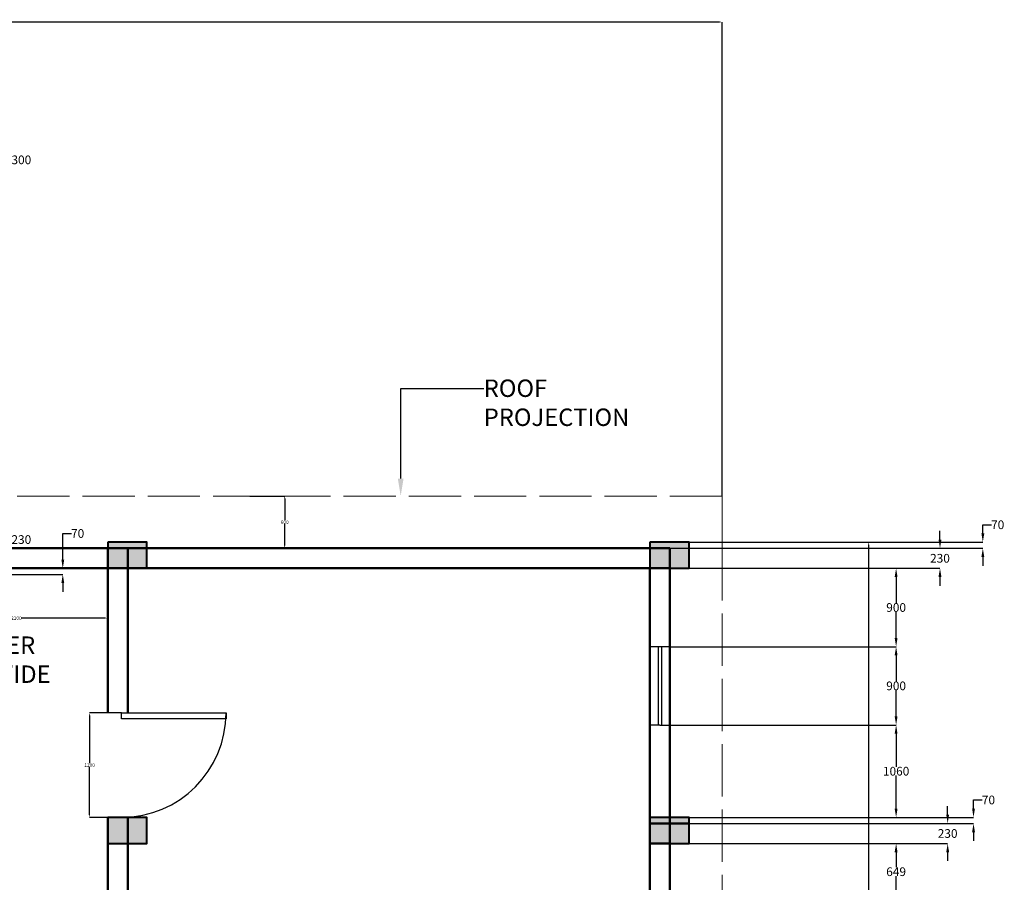
# Model space of a CAD drawing. Units: millimetres. Extents: x -17156 to 39375, y -45872 to -24892.
# Tile 11 of 12: x 5351 to 16665, y -35444 to -25539. Entities that reach past the tile are written whole.
import ezdxf
from ezdxf import colors
from ezdxf.entities.mleader import LeaderData, LeaderLine
from ezdxf.math import Vec2, Vec3

# ---------------------------------------------------------------- set-up
doc = ezdxf.new("R2010")
doc.units = ezdxf.units.MM
doc.header["$MEASUREMENT"] = 0
doc.linetypes.add('ACAD_ISO02W100', pattern=[15, 12, -3])
for name, color, linetype, lineweight in [('A-ANNO-DIMS', 2, 'Continuous', 18), ('A-ANNO-TEXT', 4, 'Continuous', 18), ('A-AREA-IDEN', 4, 'Continuous', 25), ('A-COLS', 7, 'Continuous', 40), ('A-ROOF-OVHD', 8, 'ACAD_ISO02W100', 18), ('DOORS', 6, 'Continuous', 25), ('WALLS', 5, 'Continuous', 50), ('WINDOW', 240, 'Continuous', 25)]:
    doc.layers.add(name, color=color, linetype=linetype, lineweight=lineweight)
doc.styles.get("Standard").update_dxf_attribs({"font": 'arial.ttf'})
doc.dimstyles.get("Standard").update_dxf_attribs({"dimtxt": 40, "dimasz": 30.18, "dimexe": 0, "dimexo": 0.0625, "dimgap": 0.09, "dimtad": 0, "dimtih": 1, "dimtoh": 1, "dimdec": 0, "dimzin": 0, "dimdsep": 46, "dimtxsty": 'Standard', "dimcen": 0.09, "dimadec": 0, "dimazin": 0, "dimtfac": 1, "dimtdec": 0, "dimtofl": 0, "dimtmove": 0, "dimatfit": 3, "dimfxl": 1, "dimtolj": 1, "dimtzin": 0, "dimarcsym": 0})

# ---------------------------------------------------------------- blocks, each defined once
blk = doc.blocks.new('*U8')
for p, q in [((-750, 0), (-750, 100)), ((0, 0), (0, 100))]:
    blk.add_line(p, q)
blk.add_lwpolyline([(0, 0), (0, -750), (-43.75, -750), (-43.75, 0)], close=True)
blk.add_arc((0, 0), 750, 180, 270)
blk = doc.blocks.new('*D44')
at = {"layer": 'A-ANNO-DIMS', "color": 0, "lineweight": -2, "transparency": 16777216}
for p, q in [((13043, -34998), (15422, -34998)), ((15422, -35098), (15422, -35271)), ((15422, -35547), (15422, -35374)), ((12823, -35647), (15422, -35647))]:
    blk.add_line(p, q, dxfattribs=at)
at = {"layer": 'A-ANNO-DIMS', "color": 0, "lineweight": 100, "transparency": 16777216}
for points in [[(15405, -35098), (15438, -35098), (15422, -34998)], [(15405, -35547), (15438, -35547), (15422, -35647)]]:
    blk.add_solid(points, dxfattribs=at)
at = {"layer": 'Defpoints', "color": 0, "lineweight": 100, "transparency": 16777216}
for p in [(13043, -34998), (15422, -34998), (12823, -35647)]:
    blk.add_point(p, dxfattribs=at)
at = {"layer": 'A-ANNO-DIMS', "color": 0, "transparency": 16777216, "insert": (15422, -35322), "char_height": 100, "attachment_point": 5}
blk.add_mtext('\\A1;649', dxfattribs=at)
blk = doc.blocks.new('*D45')
at = {"layer": 'A-ANNO-DIMS', "color": 0, "lineweight": -2, "transparency": 16777216}
for p, q in [((16014, -34668), (16014, -34568)), ((13043, -34768), (16014, -34768)), ((13043, -34998), (16014, -34998)), ((16014, -35098), (16014, -35198))]:
    blk.add_line(p, q, dxfattribs=at)
at = {"layer": 'A-ANNO-DIMS', "color": 0, "lineweight": 100, "transparency": 16777216}
for points in [[(15998, -34668), (16031, -34668), (16014, -34768)], [(15998, -35098), (16031, -35098), (16014, -34998)]]:
    blk.add_solid(points, dxfattribs=at)
at = {"layer": 'Defpoints', "color": 0, "lineweight": 100, "transparency": 16777216}
for p in [(13043, -34768), (16014, -34768), (13043, -34998)]:
    blk.add_point(p, dxfattribs=at)
at = {"layer": 'A-ANNO-DIMS', "color": 0, "transparency": 16777216, "insert": (16014, -34883), "char_height": 100, "attachment_point": 5}
blk.add_mtext('\\A1;230', dxfattribs=at)
blk = doc.blocks.new('*D46')
at = {"layer": 'A-ANNO-DIMS', "color": 0, "lineweight": -2, "transparency": 16777216}
for p, q in [((16311, -34598), (16311, -34498)), ((16311, -34498), (16411, -34498)), ((13043, -34698), (16311, -34698)), ((13043, -34768), (16311, -34768)), ((16311, -34868), (16311, -34968))]:
    blk.add_line(p, q, dxfattribs=at)
at = {"layer": 'A-ANNO-DIMS', "color": 0, "lineweight": 100, "transparency": 16777216}
for points in [[(16295, -34598), (16328, -34598), (16311, -34698)], [(16295, -34868), (16328, -34868), (16311, -34768)]]:
    blk.add_solid(points, dxfattribs=at)
at = {"layer": 'Defpoints', "color": 0, "lineweight": 100, "transparency": 16777216}
for p in [(13043, -34698), (16311, -34698), (13043, -34768)]:
    blk.add_point(p, dxfattribs=at)
at = {"layer": 'A-ANNO-DIMS', "color": 0, "transparency": 16777216, "insert": (16483, -34498), "char_height": 100, "attachment_point": 5}
blk.add_mtext('\\A1;70', dxfattribs=at)
blk = doc.blocks.new('*D47')
at = {"layer": 'A-ANNO-DIMS', "color": 0, "lineweight": -2, "transparency": 16777216}
for p, q in [((12823, -33638), (15422, -33638)), ((15422, -33738), (15422, -34117)), ((15422, -34598), (15422, -34219)), ((13043, -34698), (15422, -34698))]:
    blk.add_line(p, q, dxfattribs=at)
at = {"layer": 'A-ANNO-DIMS', "color": 0, "lineweight": 100, "transparency": 16777216}
for points in [[(15405, -33738), (15438, -33738), (15422, -33638)], [(15405, -34598), (15438, -34598), (15422, -34698)]]:
    blk.add_solid(points, dxfattribs=at)
at = {"layer": 'Defpoints', "color": 0, "lineweight": 100, "transparency": 16777216}
for p in [(12823, -33638), (15422, -33638), (13043, -34698)]:
    blk.add_point(p, dxfattribs=at)
at = {"layer": 'A-ANNO-DIMS', "color": 0, "transparency": 16777216, "insert": (15422, -34168), "char_height": 100, "attachment_point": 5}
blk.add_mtext('\\A1;1060', dxfattribs=at)
blk = doc.blocks.new('*D48')
at = {"layer": 'A-ANNO-DIMS', "color": 0, "lineweight": -2, "transparency": 16777216}
for p, q in [((12823, -32738), (15422, -32738)), ((15422, -32838), (15422, -33136)), ((15422, -33538), (15422, -33239)), ((12823, -33638), (15422, -33638))]:
    blk.add_line(p, q, dxfattribs=at)
at = {"layer": 'A-ANNO-DIMS', "color": 0, "lineweight": 100, "transparency": 16777216}
for points in [[(15405, -32838), (15438, -32838), (15422, -32738)], [(15405, -33538), (15438, -33538), (15422, -33638)]]:
    blk.add_solid(points, dxfattribs=at)
at = {"layer": 'Defpoints', "color": 0, "lineweight": 100, "transparency": 16777216}
for p in [(12823, -32738), (15422, -32738), (12823, -33638)]:
    blk.add_point(p, dxfattribs=at)
at = {"layer": 'A-ANNO-DIMS', "color": 0, "transparency": 16777216, "insert": (15422, -33188), "char_height": 100, "attachment_point": 5}
blk.add_mtext('\\A1;900', dxfattribs=at)
blk = doc.blocks.new('*D49')
at = {"layer": 'A-ANNO-DIMS', "color": 0, "lineweight": -2, "transparency": 16777216}
for p, q in [((13043, -31838), (15422, -31838)), ((15422, -31938), (15422, -32237)), ((15422, -32638), (15422, -32339)), ((12823, -32738), (15422, -32738))]:
    blk.add_line(p, q, dxfattribs=at)
at = {"layer": 'A-ANNO-DIMS', "color": 0, "lineweight": 100, "transparency": 16777216}
for points in [[(15405, -31938), (15438, -31938), (15422, -31838)], [(15405, -32638), (15438, -32638), (15422, -32738)]]:
    blk.add_solid(points, dxfattribs=at)
at = {"layer": 'Defpoints', "color": 0, "lineweight": 100, "transparency": 16777216}
for p in [(13043, -31838), (15422, -31838), (12823, -32738)]:
    blk.add_point(p, dxfattribs=at)
at = {"layer": 'A-ANNO-DIMS', "color": 0, "transparency": 16777216, "insert": (15422, -32288), "char_height": 100, "attachment_point": 5}
blk.add_mtext('\\A1;900', dxfattribs=at)
blk = doc.blocks.new('*D50')
at = {"layer": 'A-ANNO-DIMS', "color": 0, "lineweight": -2, "transparency": 16777216}
for p, q in [((15926, -31508), (15926, -31408)), ((12823, -31608), (15926, -31608)), ((13043, -31838), (15926, -31838)), ((15926, -31938), (15926, -32038))]:
    blk.add_line(p, q, dxfattribs=at)
at = {"layer": 'A-ANNO-DIMS', "color": 0, "lineweight": 100, "transparency": 16777216}
for points in [[(15909, -31508), (15943, -31508), (15926, -31608)], [(15909, -31938), (15943, -31938), (15926, -31838)]]:
    blk.add_solid(points, dxfattribs=at)
at = {"layer": 'Defpoints', "color": 0, "lineweight": 100, "transparency": 16777216}
for p in [(12823, -31608), (15926, -31608), (13043, -31838)]:
    blk.add_point(p, dxfattribs=at)
at = {"layer": 'A-ANNO-DIMS', "color": 0, "transparency": 16777216, "insert": (15926, -31723), "char_height": 100, "attachment_point": 5}
blk.add_mtext('\\A1;230', dxfattribs=at)
blk = doc.blocks.new('*D51')
at = {"layer": 'A-ANNO-DIMS', "color": 0, "lineweight": -2, "transparency": 16777216}
for p, q in [((16418, -31438), (16418, -31338)), ((16418, -31338), (16518, -31338)), ((13043, -31538), (16418, -31538)), ((12823, -31608), (16418, -31608)), ((16418, -31708), (16418, -31808))]:
    blk.add_line(p, q, dxfattribs=at)
at = {"layer": 'A-ANNO-DIMS', "color": 0, "lineweight": 100, "transparency": 16777216}
for points in [[(16402, -31438), (16435, -31438), (16418, -31538)], [(16402, -31708), (16435, -31708), (16418, -31608)]]:
    blk.add_solid(points, dxfattribs=at)
at = {"layer": 'Defpoints', "color": 0, "lineweight": 100, "transparency": 16777216}
for p in [(13043, -31538), (16418, -31538), (12823, -31608)]:
    blk.add_point(p, dxfattribs=at)
at = {"layer": 'A-ANNO-DIMS', "color": 0, "transparency": 16777216, "insert": (16589, -31338), "char_height": 100, "attachment_point": 5}
blk.add_mtext('\\A1;70', dxfattribs=at)
blk = doc.blocks.new('*D73')
at = {"layer": 'A-ANNO-DIMS', "color": 0, "lineweight": -2, "transparency": 16777216}
for p, q in [((5846, -31738), (5846, -31438)), ((5846, -31438), (5946, -31438)), ((4493, -31838), (5846, -31838)), ((4493, -31908), (5846, -31908)), ((5846, -32008), (5846, -32108))]:
    blk.add_line(p, q, dxfattribs=at)
at = {"layer": 'A-ANNO-DIMS', "color": 0, "lineweight": 100, "transparency": 16777216}
for points in [[(5830, -31738), (5863, -31738), (5846, -31838)], [(5830, -32008), (5863, -32008), (5846, -31908)]]:
    blk.add_solid(points, dxfattribs=at)
at = {"layer": 'Defpoints', "color": 0, "lineweight": 100, "transparency": 16777216}
for p in [(4493, -31838), (5846, -31838), (4493, -31908)]:
    blk.add_point(p, dxfattribs=at)
at = {"layer": 'A-ANNO-DIMS', "color": 0, "transparency": 16777216, "insert": (6017, -31438), "char_height": 100, "attachment_point": 5}
blk.add_mtext('\\A1;70', dxfattribs=at)
blk = doc.blocks.new('*D74')
at = {"layer": 'A-ANNO-DIMS', "color": 0, "lineweight": -2, "transparency": 16777216}
for p, q in [((5159, -31608), (5159, -31508)), ((5159, -31508), (5259, -31508)), ((4493, -31608), (5159, -31608)), ((5159, -31738), (5159, -31708)), ((4493, -31838), (5159, -31838))]:
    blk.add_line(p, q, dxfattribs=at)
at = {"layer": 'A-ANNO-DIMS', "color": 0, "lineweight": 100, "transparency": 16777216}
for points in [[(5143, -31708), (5176, -31708), (5159, -31608)], [(5143, -31738), (5176, -31738), (5159, -31838)]]:
    blk.add_solid(points, dxfattribs=at)
at = {"layer": 'Defpoints', "color": 0, "lineweight": 100, "transparency": 16777216}
for p in [(4493, -31608), (5159, -31608), (4493, -31838)]:
    blk.add_point(p, dxfattribs=at)
at = {"layer": 'A-ANNO-DIMS', "color": 0, "transparency": 16777216, "insert": (5370, -31508), "char_height": 100, "attachment_point": 5}
blk.add_mtext('\\A1;230', dxfattribs=at)
blk = doc.blocks.new('*D76')
at = {"layer": 'A-ANNO-DIMS', "color": 0, "lineweight": -2, "transparency": 16777216}
for p, q in [((5159, -27248), (5159, -27148)), ((5159, -27148), (5259, -27148)), ((4493, -27248), (5159, -27248)), ((5159, -27448), (5159, -27348)), ((4493, -27548), (5159, -27548))]:
    blk.add_line(p, q, dxfattribs=at)
at = {"layer": 'A-ANNO-DIMS', "color": 0, "lineweight": 100, "transparency": 16777216}
for points in [[(5143, -27348), (5176, -27348), (5159, -27248)], [(5143, -27448), (5176, -27448), (5159, -27548)]]:
    blk.add_solid(points, dxfattribs=at)
at = {"layer": 'Defpoints', "color": 0, "lineweight": 100, "transparency": 16777216}
for p in [(4493, -27248), (5159, -27248), (4493, -27548)]:
    blk.add_point(p, dxfattribs=at)
at = {"layer": 'A-ANNO-DIMS', "color": 0, "transparency": 16777216, "insert": (5370, -27148), "char_height": 100, "attachment_point": 5}
blk.add_mtext('\\A1;300', dxfattribs=at)
blk = doc.blocks.new('*D107')
at = {"layer": 'A-ANNO-DIMS', "color": 0, "lineweight": -2, "transparency": 16777216}
for p, q in [((4263, -31890), (4263, -32410)), ((6363, -31890), (6363, -32410)), ((4293, -32410), (5253, -32410)), ((6332, -32410), (5373, -32410))]:
    blk.add_line(p, q, dxfattribs=at)
at = {"layer": 'A-ANNO-DIMS', "color": 0, "lineweight": 100, "transparency": 16777216}
for points in [[(4293, -32405), (4293, -32415), (4263, -32410)], [(6332, -32405), (6332, -32415), (6363, -32410)]]:
    blk.add_solid(points, dxfattribs=at)
at = {"layer": 'Defpoints', "color": 0, "lineweight": 100, "transparency": 16777216}
for p in [(4263, -31890), (6363, -31890), (6363, -32410)]:
    blk.add_point(p, dxfattribs=at)
at = {"layer": 'A-ANNO-DIMS', "color": 0, "transparency": 16777216, "insert": (5313, -32410), "char_height": 40, "attachment_point": 5}
blk.add_mtext('\\A1;2100', dxfattribs=at)
blk = doc.blocks.new('*D110')
at = {"layer": 'A-ANNO-DIMS', "color": 0, "lineweight": -2, "transparency": 16777216}
for p, q in [((7996, -31008), (8396, -31008)), ((8396, -31038), (8396, -31287)), ((8396, -31578), (8396, -31328)), ((7996, -31608), (8396, -31608))]:
    blk.add_line(p, q, dxfattribs=at)
at = {"layer": 'A-ANNO-DIMS', "color": 0, "lineweight": 100, "transparency": 16777216}
for points in [[(8391, -31038), (8401, -31038), (8396, -31008)], [(8391, -31578), (8401, -31578), (8396, -31608)]]:
    blk.add_solid(points, dxfattribs=at)
at = {"layer": 'Defpoints', "color": 0, "lineweight": 100, "transparency": 16777216}
for p in [(7996, -31008), (7996, -31608), (8396, -31608)]:
    blk.add_point(p, dxfattribs=at)
at = {"layer": 'A-ANNO-DIMS', "color": 0, "transparency": 16777216, "insert": (8396, -31308), "char_height": 40, "attachment_point": 5}
blk.add_mtext('\\A1;600', dxfattribs=at)
blk = doc.blocks.new('*D113')
at = {"layer": 'A-ANNO-DIMS', "color": 0, "lineweight": -2, "transparency": 16777216}
for p, q in [((6363, -33498), (6155, -33498)), ((6155, -33528), (6155, -34077)), ((6155, -34668), (6155, -34118)), ((6363, -34698), (6155, -34698))]:
    blk.add_line(p, q, dxfattribs=at)
at = {"layer": 'A-ANNO-DIMS', "color": 0, "lineweight": 100, "transparency": 16777216}
for points in [[(6150, -33528), (6160, -33528), (6155, -33498)], [(6150, -34668), (6160, -34668), (6155, -34698)]]:
    blk.add_solid(points, dxfattribs=at)
at = {"layer": 'Defpoints', "color": 0, "lineweight": 100, "transparency": 16777216}
for p in [(6363, -33498), (6155, -34698), (6363, -34698)]:
    blk.add_point(p, dxfattribs=at)
at = {"layer": 'A-ANNO-DIMS', "color": 0, "transparency": 16777216, "insert": (6155, -34098), "char_height": 40, "attachment_point": 5}
blk.add_mtext('\\A1;1200', dxfattribs=at)
blk = doc.blocks.new('WIN-900x230')
for p, q in [((0, 900), (230, 900)), ((95, 900), (95, 0)), ((135, 900), (135, 0)), ((115, 0), (0, 0)), ((115, 0), (230, 0))]:
    blk.add_line(p, q)
blk = doc.blocks.new('COL-450x300')
h = blk.add_hatch(color=256)
h.dxf.hatch_style = 1
h.paths.add_polyline_path([(0, 300), (0, 0), (450, 0), (450, 300)])
blk.add_lwpolyline([(0, 300), (0, 0), (450, 0), (450, 300)], close=True)
blk = doc.blocks.new('*D144')
at = {"layer": 'A-ANNO-DIMS', "color": 0, "lineweight": -2, "transparency": 16777216}
for p, q in [((-15397, -31008), (-15397, -25565)), ((-15367, -25565), (-1063, -25565)), ((13392, -25565), (-912, -25565)), ((13423, -31008), (13423, -25565))]:
    blk.add_line(p, q, dxfattribs=at)
at = {"layer": 'A-ANNO-DIMS', "color": 0, "lineweight": 100, "transparency": 16777216}
for points in [[(-15367, -25560), (-15367, -25570), (-15397, -25565)], [(13392, -25560), (13392, -25570), (13423, -25565)]]:
    blk.add_solid(points, dxfattribs=at)
at = {"layer": 'Defpoints', "color": 0, "lineweight": 100, "transparency": 16777216}
for p in [(13423, -25565), (-15397, -31008), (13423, -31008)]:
    blk.add_point(p, dxfattribs=at)
at = {"layer": 'A-ANNO-DIMS', "color": 0, "transparency": 16777216, "insert": (-987, -25565), "char_height": 40, "attachment_point": 5}
blk.add_mtext('\\A1;28820', dxfattribs=at)
blk = doc.blocks.new('*D147')
at = {"layer": 'A-ANNO-DIMS', "color": 0, "lineweight": -2, "transparency": 16777216}
for p, q in [((13043, -31538), (15106, -31538)), ((15106, -31568), (15106, -37115)), ((15106, -42703), (15106, -37156)), ((13043, -42733), (15106, -42733))]:
    blk.add_line(p, q, dxfattribs=at)
at = {"layer": 'A-ANNO-DIMS', "color": 0, "lineweight": 100, "transparency": 16777216}
for points in [[(15101, -31568), (15111, -31568), (15106, -31538)], [(15101, -42703), (15111, -42703), (15106, -42733)]]:
    blk.add_solid(points, dxfattribs=at)
at = {"layer": 'Defpoints', "color": 0, "lineweight": 100, "transparency": 16777216}
for p in [(13043, -31538), (15106, -31538), (13043, -42733)]:
    blk.add_point(p, dxfattribs=at)
at = {"layer": 'A-ANNO-DIMS', "color": 0, "transparency": 16777216, "insert": (15106, -37135), "char_height": 40, "attachment_point": 5}
blk.add_mtext('\\A1;11195', dxfattribs=at)

msp = doc.modelspace()

# ---------------------------------------------------------------- linework, layer by layer
at = {"layer": 'A-ROOF-OVHD', "ltscale": 50}
for p, q in [((13422.65, -31007.85), (3662.65, -31007.85)), ((13422.65, -31607.85), (13422.65, -31007.85)), ((13422.65, -31607.85), (13422.65, -42662.85))]:
    msp.add_line(p, q, dxfattribs=at)
at = {"layer": 'WALLS'}
for p, q in [((12822.65, -31607.85), (4262.65, -31607.85)), ((6362.65, -31607.85), (6362.65, -33497.85)), ((6592.65, -31607.85), (6592.65, -33497.85)), ((12822.65, -31607.85), (12822.65, -42662.85)), ((12822.65, -31837.85), (4192.65, -31837.85)), ((12592.65, -31837.85), (12592.65, -42432.85)), ((6362.65, -34697.85), (6362.65, -37112.85)), ((6592.65, -34697.85), (6592.65, -37114.89)), ((13042.65, -34767.85), (12592.65, -34767.85)), ((12822.65, -34997.85), (12592.65, -34997.85))]:
    msp.add_line(p, q, dxfattribs=at)

# ---------------------------------------------------------------- block references
at = {"layer": 'A-COLS'}
for p in [(6362.65, -31837.85), (12592.65, -31837.85), (12592.65, -31837.85), (6362.65, -34997.85), (12592.65, -34997.85), (12592.65, -34997.85)]:
    msp.add_blockref('COL-450x300', p, dxfattribs=at)
at = {"layer": 'DOORS', "xscale": 1.6, "yscale": 1.6, "zscale": 1.6, "rotation": 90}
msp.add_blockref('*U8', (6522.65, -33497.85), dxfattribs=at)
at = {"layer": 'WINDOW'}
msp.add_blockref('WIN-900x230', (12592.65, -33637.56), dxfattribs=at)

# ---------------------------------------------------------------- texts
at = {"layer": 'A-AREA-IDEN', "insert": (5038.26, -32620.61), "char_height": 200, "attachment_point": 1}
msp.add_mtext_dynamic_manual_height_columns('{VER WIDE}', width=660.3665, gutter_width=1, heights=[0], dxfattribs=at)

# ---------------------------------------------------------------- dimensions: what is measured, and where the dimension line sits
at = {"layer": 'A-ANNO-DIMS'}
dim = msp.add_linear_dim(base=(13422.65, -25564.85), p1=(-15397.35, -31007.85), p2=(13422.65, -31007.85), dimstyle='Standard', override={"dimdec": 0, "dimlfac": 1, "dimrnd": 0, "dimzin": 0, "dimdsep": 46, "dimlunit": 2}, dxfattribs=at)
dim.commit()
dim.dimension.update_dxf_attribs({"geometry": '*D144', "text_midpoint": (-987.35, -25564.85)})
for base, p1, p2, angle, override, picture, middle in [((5159.25, -27247.85), (4492.65, -27547.85), (4492.65, -27247.85), 270, {"dimtxt": 100, "dimasz": 100, "dimclrd": 0, "dimclre": 0, "dimclrt": 0}, '*D76', (5369.61, -27147.85)), ((8395.87, -31607.85), (7996.04, -31007.85), (7996.04, -31607.85), 90, {"dimclrd": 0, "dimclre": 0, "dimclrt": 0}, '*D110', (8395.87, -31307.85)), ((16418.21, -31537.85), (12822.65, -31607.85), (13042.65, -31537.85), 270, {"dimtxt": 100, "dimasz": 100, "dimclrd": 0, "dimclre": 0, "dimclrt": 0}, '*D51', (16589.34, -31337.85)), ((5159.25, -31607.85), (4492.65, -31837.85), (4492.65, -31607.85), 270, {"dimtxt": 100, "dimasz": 100, "dimclrd": 0, "dimclre": 0, "dimclrt": 0}, '*D74', (5370.49, -31507.85)), ((15105.65, -31537.85), (13042.65, -42732.85), (13042.65, -31537.85), 90, {"dimdec": 0, "dimlfac": 1, "dimrnd": 0, "dimzin": 0, "dimdsep": 46, "dimlunit": 2}, '*D147', (15105.65, -37135.35)), ((15421.51, -31837.85), (12822.65, -32737.56), (13042.65, -31837.85), 270, {"dimtxt": 100, "dimasz": 100, "dimclrd": 0, "dimclre": 0, "dimclrt": 0}, '*D49', (15421.51, -32287.7)), ((15421.51, -32737.56), (12822.65, -33637.56), (12822.65, -32737.56), 270, {"dimtxt": 100, "dimasz": 100, "dimclrd": 0, "dimclre": 0, "dimclrt": 0}, '*D48', (15421.51, -33187.56)), ((6155.4, -34697.85), (6362.65, -33497.85), (6362.65, -34697.85), 90, {"dimclrd": 0, "dimclre": 0, "dimclrt": 0}, '*D113', (6155.4, -34097.85)), ((15421.51, -33637.56), (13042.65, -34697.85), (12822.65, -33637.56), 270, {"dimtxt": 100, "dimasz": 100, "dimclrd": 0, "dimclre": 0, "dimclrt": 0}, '*D47', (15421.51, -34167.7)), ((16311.43, -34697.85), (13042.65, -34767.85), (13042.65, -34697.85), 270, {"dimtxt": 100, "dimasz": 100, "dimclrd": 0, "dimclre": 0, "dimclrt": 0}, '*D46', (16482.57, -34497.85)), ((15421.51, -34997.85), (12822.65, -35646.91), (13042.65, -34997.85), 270, {"dimtxt": 100, "dimasz": 100, "dimclrd": 0, "dimclre": 0, "dimclrt": 0}, '*D44', (15421.51, -35322.38))]:
    dim = msp.add_linear_dim(base=base, p1=p1, p2=p2, angle=angle, dimstyle='Standard', override=override, dxfattribs=at)
    dim.commit()
    dim.dimension.update_dxf_attribs({"geometry": picture, "text_midpoint": middle})
for base, p1, p2, picture, middle in [((5846.23, -31837.85), (4492.65, -31907.85), (4492.65, -31837.85), '*D73', (6017.36, -31437.85)), ((15925.93, -31607.85), (13042.65, -31837.85), (12822.65, -31607.85), '*D50', (15925.93, -31722.85)), ((16014.38, -34767.85), (13042.65, -34997.85), (13042.65, -34767.85), '*D45', (16014.38, -34882.85))]:
    dim = msp.add_linear_dim(base=base, p1=p1, p2=p2, angle=270, dimstyle='Standard', override={"dimtxt": 100, "dimasz": 100, "dimclrd": 0, "dimclre": 0, "dimclrt": 0}, dxfattribs=at)
    dim.commit()
    dim.dimension.update_dxf_attribs({"geometry": picture, "text_midpoint": middle, "dimtype": 160})
dim = msp.add_linear_dim(base=(6362.65, -32410.02), p1=(4262.65, -31890.1), p2=(6362.65, -31890.1), dimstyle='Standard', override={"dimclrd": 0, "dimclre": 0, "dimclrt": 0}, dxfattribs=at)
dim.commit()
dim.dimension.update_dxf_attribs({"geometry": '*D107', "text_midpoint": (5312.65, -32410.02), "dimtype": 160})

# ---------------------------------------------------------------- leaders
at = {"layer": 'A-ANNO-TEXT'}
ml = msp.add_multileader_mtext('Standard', dxfattribs=at)
ml.set_content('{\\C4;ROOF \\PPROJECTION}', color=256)
ml.set_leader_properties()
ml.build(insert=Vec2(0, 0))
ml.multileader.update_dxf_attribs({"dogleg_length": 0.36, "arrow_head_size": 200})
ctx = ml.context
ctx.base_point, ctx.char_height, ctx.arrow_head_size, ctx.landing_gap_size, ctx.plane_origin = Vec3(10683.31, -29771.89), 200, 200, 0.09, Vec3(9728.96, -31007.85)
notes = []
notes.append((ctx, [(0, (1, 1, 0), (10682.95, -29771.89), (1, 0), 0.36, [(0, [(9728.96, -31007.85), (9728.96, -29771.89)], 0, [])])]))
ctx.mtext.insert, ctx.mtext.flow_direction = Vec3(10683.4, -29670.19), 5
for ctx, leaders in notes:
    for number, flags, end, landing, length, lines in leaders:
        leader = LeaderData()
        leader.index, (leader.has_last_leader_line, leader.has_dogleg_vector, leader.attachment_direction) = number, flags
        leader.last_leader_point, leader.dogleg_vector, leader.dogleg_length = Vec3(end), Vec3(landing), length
        for number, points, colour, breaks in lines:
            line = LeaderLine()
            line.index, line.vertices, line.color, line.breaks = number, Vec3.list(points), colors.encode_raw_color(colour), breaks
            leader.lines.append(line)
        ctx.leaders.append(leader)

doc.saveas('drawing.dxf')
